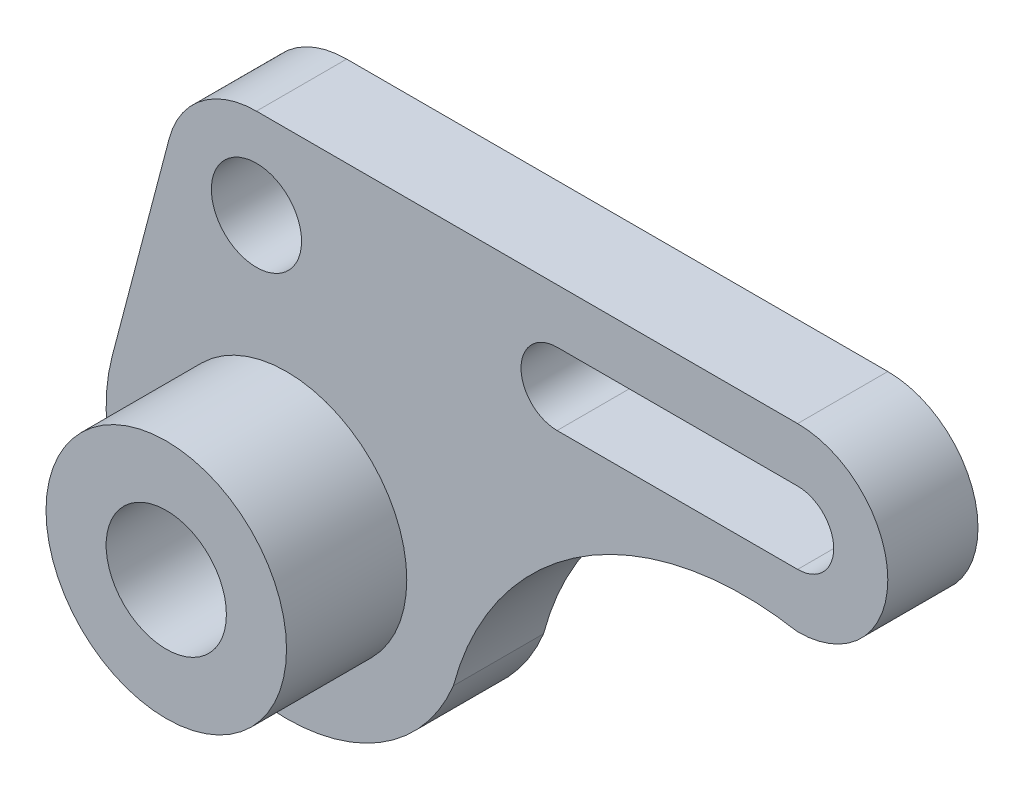
ISO-10303-21;
HEADER;
FILE_DESCRIPTION(('STEP AP214'),'2;1');
FILE_NAME('part.step','',(''),(''),'','','');
FILE_SCHEMA(('AUTOMOTIVE_DESIGN { 1 0 10303 214 1 1 1 1 }'));
ENDSEC;
DATA;
#1=APPLICATION_CONTEXT('core data for automotive mechanical design processes');
#2=APPLICATION_PROTOCOL_DEFINITION('international standard','automotive_design',2000,#1);
#3=PRODUCT_CONTEXT('',#1,'mechanical');
#4=PRODUCT('Part','Part','',(#3));
#5=PRODUCT_RELATED_PRODUCT_CATEGORY('part','',(#4));
#6=PRODUCT_DEFINITION_FORMATION('','',#4);
#7=PRODUCT_DEFINITION_CONTEXT('part definition',#1,'design');
#8=PRODUCT_DEFINITION('design','',#6,#7);
#9=PRODUCT_DEFINITION_SHAPE('','',#8);
#10=(LENGTH_UNIT() NAMED_UNIT(*) SI_UNIT(.MILLI.,.METRE.));
#11=(NAMED_UNIT(*) PLANE_ANGLE_UNIT() SI_UNIT($,.RADIAN.));
#12=(NAMED_UNIT(*) SI_UNIT($,.STERADIAN.) SOLID_ANGLE_UNIT());
#13=UNCERTAINTY_MEASURE_WITH_UNIT(LENGTH_MEASURE(1.E-05),#10,'distance_accuracy_value','');
#14=(GEOMETRIC_REPRESENTATION_CONTEXT(3) GLOBAL_UNCERTAINTY_ASSIGNED_CONTEXT((#13)) GLOBAL_UNIT_ASSIGNED_CONTEXT((#10,
#11,#12)) REPRESENTATION_CONTEXT('',''));
#15=CARTESIAN_POINT('',(0.,0.,0.));
#16=DIRECTION('',(0.,0.,1.));
#17=DIRECTION('',(1.,0.,0.));
#18=AXIS2_PLACEMENT_3D('',#15,#16,#17);
#19=CARTESIAN_POINT('',(105.,-15.,15.));
#20=DIRECTION('',(0.,0.,-1.));
#21=DIRECTION('',(-1.,0.,0.));
#22=AXIS2_PLACEMENT_3D('',#19,#20,#21);
#23=CYLINDRICAL_SURFACE('',#22,15.);
#24=CARTESIAN_POINT('',(105.,-15.,0.));
#25=DIRECTION('',(0.,0.,1.));
#26=DIRECTION('',(1.,0.,0.));
#27=AXIS2_PLACEMENT_3D('',#24,#25,#26);
#28=CIRCLE('',#27,15.);
#29=CARTESIAN_POINT('',(105.,-30.,0.));
#30=VERTEX_POINT('',#29);
#31=CARTESIAN_POINT('',(105.,0.,0.));
#32=VERTEX_POINT('',#31);
#33=EDGE_CURVE('E175',#30,#32,#28,.T.);
#34=ORIENTED_EDGE('',*,*,#33,.T.);
#35=DIRECTION('',(0.,0.,-1.));
#36=VECTOR('',#35,1.);
#37=CARTESIAN_POINT('',(105.,0.,15.));
#38=LINE('',#37,#36);
#39=CARTESIAN_POINT('',(105.,0.,15.));
#40=VERTEX_POINT('',#39);
#41=EDGE_CURVE('E11',#40,#32,#38,.T.);
#42=ORIENTED_EDGE('',*,*,#41,.F.);
#43=CARTESIAN_POINT('',(105.,-15.,15.));
#44=DIRECTION('',(0.,0.,1.));
#45=DIRECTION('',(1.,0.,0.));
#46=AXIS2_PLACEMENT_3D('',#43,#44,#45);
#47=CIRCLE('',#46,15.);
#48=CARTESIAN_POINT('',(105.,-30.,15.));
#49=VERTEX_POINT('',#48);
#50=EDGE_CURVE('E178',#49,#40,#47,.T.);
#51=ORIENTED_EDGE('',*,*,#50,.F.);
#52=DIRECTION('',(0.,0.,-1.));
#53=VECTOR('',#52,1.);
#54=CARTESIAN_POINT('',(105.,-30.,15.));
#55=LINE('',#54,#53);
#56=EDGE_CURVE('E188',#49,#30,#55,.T.);
#57=ORIENTED_EDGE('',*,*,#56,.T.);
#58=EDGE_LOOP('',(#34,#42,#51,#57));
#59=FACE_BOUND('',#58,.T.);
#60=ADVANCED_FACE('F44',(#59),#23,.T.);
#61=CARTESIAN_POINT('',(15.0000000000001,0.,15.));
#62=DIRECTION('',(0.,-1.,0.));
#63=DIRECTION('',(0.,0.,-1.));
#64=AXIS2_PLACEMENT_3D('',#61,#62,#63);
#65=PLANE('',#64);
#66=DIRECTION('',(-1.,0.,0.));
#67=VECTOR('',#66,1.);
#68=CARTESIAN_POINT('',(15.0000000000001,0.,0.));
#69=LINE('',#68,#67);
#70=CARTESIAN_POINT('',(15.0000000000001,0.,0.));
#71=VERTEX_POINT('',#70);
#72=EDGE_CURVE('E191',#32,#71,#69,.T.);
#73=ORIENTED_EDGE('',*,*,#72,.T.);
#74=DIRECTION('',(0.,0.,-1.));
#75=VECTOR('',#74,1.);
#76=CARTESIAN_POINT('',(15.0000000000001,0.,15.));
#77=LINE('',#76,#75);
#78=CARTESIAN_POINT('',(15.0000000000001,0.,15.));
#79=VERTEX_POINT('',#78);
#80=EDGE_CURVE('E55',#79,#71,#77,.T.);
#81=ORIENTED_EDGE('',*,*,#80,.F.);
#82=DIRECTION('',(-1.,0.,0.));
#83=VECTOR('',#82,1.);
#84=CARTESIAN_POINT('',(15.0000000000001,0.,15.));
#85=LINE('',#84,#83);
#86=EDGE_CURVE('E179',#40,#79,#85,.T.);
#87=ORIENTED_EDGE('',*,*,#86,.F.);
#88=ORIENTED_EDGE('',*,*,#41,.T.);
#89=EDGE_LOOP('',(#73,#81,#87,#88));
#90=FACE_BOUND('',#89,.T.);
#91=ADVANCED_FACE('F239',(#90),#65,.F.);
#92=CARTESIAN_POINT('',(15.,-15.,15.));
#93=DIRECTION('',(0.,0.,-1.));
#94=DIRECTION('',(-1.,0.,0.));
#95=AXIS2_PLACEMENT_3D('',#92,#93,#94);
#96=CYLINDRICAL_SURFACE('',#95,15.);
#97=CARTESIAN_POINT('',(15.,-15.,0.));
#98=DIRECTION('',(0.,0.,1.));
#99=DIRECTION('',(1.,0.,0.));
#100=AXIS2_PLACEMENT_3D('',#97,#98,#99);
#101=CIRCLE('',#100,15.);
#102=CARTESIAN_POINT('',(0.492341956526993,-11.1884572554341,0.));
#103=VERTEX_POINT('',#102);
#104=EDGE_CURVE('E192',#71,#103,#101,.T.);
#105=ORIENTED_EDGE('',*,*,#104,.T.);
#106=DIRECTION('',(0.,0.,-1.));
#107=VECTOR('',#106,1.);
#108=CARTESIAN_POINT('',(0.492341956526993,-11.1884572554341,15.));
#109=LINE('',#108,#107);
#110=CARTESIAN_POINT('',(0.492341956526993,-11.1884572554341,15.));
#111=VERTEX_POINT('',#110);
#112=EDGE_CURVE('E209',#111,#103,#109,.T.);
#113=ORIENTED_EDGE('',*,*,#112,.F.);
#114=CARTESIAN_POINT('',(15.,-15.,15.));
#115=DIRECTION('',(0.,0.,1.));
#116=DIRECTION('',(1.,0.,0.));
#117=AXIS2_PLACEMENT_3D('',#114,#115,#116);
#118=CIRCLE('',#117,15.);
#119=EDGE_CURVE('E185',#79,#111,#118,.T.);
#120=ORIENTED_EDGE('',*,*,#119,.F.);
#121=ORIENTED_EDGE('',*,*,#80,.T.);
#122=EDGE_LOOP('',(#105,#113,#120,#121));
#123=FACE_BOUND('',#122,.T.);
#124=ADVANCED_FACE('F220',(#123),#96,.T.);
#125=CARTESIAN_POINT('',(-9.01531608694612,-47.3769145108682,15.));
#126=DIRECTION('',(0.9671772028982,-0.254102849637728,0.));
#127=DIRECTION('',(0.254102849637728,0.9671772028982,0.));
#128=AXIS2_PLACEMENT_3D('',#125,#126,#127);
#129=PLANE('',#128);
#130=DIRECTION('',(-0.254102849637728,-0.9671772028982,0.));
#131=VECTOR('',#130,1.);
#132=CARTESIAN_POINT('',(-9.01531608694612,-47.3769145108682,0.));
#133=LINE('',#132,#131);
#134=CARTESIAN_POINT('',(-9.01531608694612,-47.3769145108682,0.));
#135=VERTEX_POINT('',#134);
#136=EDGE_CURVE('E197',#103,#135,#133,.T.);
#137=ORIENTED_EDGE('',*,*,#136,.T.);
#138=DIRECTION('',(0.,0.,-1.));
#139=VECTOR('',#138,1.);
#140=CARTESIAN_POINT('',(-9.01531608694612,-47.3769145108682,15.));
#141=LINE('',#140,#139);
#142=CARTESIAN_POINT('',(-9.01531608694612,-47.3769145108682,15.));
#143=VERTEX_POINT('',#142);
#144=EDGE_CURVE('E210',#143,#135,#141,.T.);
#145=ORIENTED_EDGE('',*,*,#144,.F.);
#146=DIRECTION('',(-0.254102849637728,-0.9671772028982,0.));
#147=VECTOR('',#146,1.);
#148=CARTESIAN_POINT('',(-9.01531608694612,-47.3769145108682,15.));
#149=LINE('',#148,#147);
#150=EDGE_CURVE('E184',#111,#143,#149,.T.);
#151=ORIENTED_EDGE('',*,*,#150,.F.);
#152=ORIENTED_EDGE('',*,*,#112,.T.);
#153=EDGE_LOOP('',(#137,#145,#151,#152));
#154=FACE_BOUND('',#153,.T.);
#155=ADVANCED_FACE('F229',(#154),#129,.F.);
#156=CARTESIAN_POINT('',(20.,-55.,15.));
#157=DIRECTION('',(0.,0.,-1.));
#158=DIRECTION('',(-1.,0.,0.));
#159=AXIS2_PLACEMENT_3D('',#156,#157,#158);
#160=CYLINDRICAL_SURFACE('',#159,30.);
#161=CARTESIAN_POINT('',(20.,-55.,0.));
#162=DIRECTION('',(0.,0.,1.));
#163=DIRECTION('',(1.,0.,0.));
#164=AXIS2_PLACEMENT_3D('',#161,#162,#163);
#165=CIRCLE('',#164,30.);
#166=CARTESIAN_POINT('',(47.7525615192124,-66.3927753037761,0.));
#167=VERTEX_POINT('',#166);
#168=EDGE_CURVE('E200',#135,#167,#165,.T.);
#169=ORIENTED_EDGE('',*,*,#168,.T.);
#170=DIRECTION('',(0.,0.,-1.));
#171=VECTOR('',#170,1.);
#172=CARTESIAN_POINT('',(47.7525615192124,-66.3927753037761,15.));
#173=LINE('',#172,#171);
#174=CARTESIAN_POINT('',(47.7525615192124,-66.3927753037761,15.));
#175=VERTEX_POINT('',#174);
#176=EDGE_CURVE('E204',#175,#167,#173,.T.);
#177=ORIENTED_EDGE('',*,*,#176,.F.);
#178=CARTESIAN_POINT('',(20.,-55.,15.));
#179=DIRECTION('',(0.,0.,1.));
#180=DIRECTION('',(1.,0.,0.));
#181=AXIS2_PLACEMENT_3D('',#178,#179,#180);
#182=CIRCLE('',#181,30.);
#183=EDGE_CURVE('E187',#143,#175,#182,.T.);
#184=ORIENTED_EDGE('',*,*,#183,.F.);
#185=ORIENTED_EDGE('',*,*,#144,.T.);
#186=EDGE_LOOP('',(#169,#177,#184,#185));
#187=FACE_BOUND('',#186,.T.);
#188=ADVANCED_FACE('F233',(#187),#160,.T.);
#189=CARTESIAN_POINT('',(96.0848114598886,-79.1987745100858,15.));
#190=DIRECTION('',(0.,0.,-1.));
#191=DIRECTION('',(-1.,0.,0.));
#192=AXIS2_PLACEMENT_3D('',#189,#190,#191);
#193=CYLINDRICAL_SURFACE('',#192,50.);
#194=CARTESIAN_POINT('',(96.0848114598886,-79.1987745100858,0.));
#195=DIRECTION('',(0.,0.,-1.));
#196=DIRECTION('',(-1.,0.,0.));
#197=AXIS2_PLACEMENT_3D('',#194,#195,#196);
#198=CIRCLE('',#197,50.);
#199=EDGE_CURVE('E177',#167,#30,#198,.T.);
#200=ORIENTED_EDGE('',*,*,#199,.T.);
#201=ORIENTED_EDGE('',*,*,#56,.F.);
#202=CARTESIAN_POINT('',(96.0848114598886,-79.1987745100858,15.));
#203=DIRECTION('',(0.,0.,-1.));
#204=DIRECTION('',(-1.,0.,0.));
#205=AXIS2_PLACEMENT_3D('',#202,#203,#204);
#206=CIRCLE('',#205,50.);
#207=EDGE_CURVE('E190',#175,#49,#206,.T.);
#208=ORIENTED_EDGE('',*,*,#207,.F.);
#209=ORIENTED_EDGE('',*,*,#176,.T.);
#210=EDGE_LOOP('',(#200,#201,#208,#209));
#211=FACE_BOUND('',#210,.T.);
#212=ADVANCED_FACE('F244',(#211),#193,.F.);
#213=CARTESIAN_POINT('',(105.,-15.,15.));
#214=DIRECTION('',(0.,0.,1.));
#215=DIRECTION('',(1.,0.,0.));
#216=AXIS2_PLACEMENT_3D('',#213,#214,#215);
#217=PLANE('',#216);
#218=CARTESIAN_POINT('',(65.,-15.,15.));
#219=DIRECTION('',(0.,0.,1.));
#220=DIRECTION('',(1.,0.,0.));
#221=AXIS2_PLACEMENT_3D('',#218,#219,#220);
#222=CIRCLE('',#221,6.);
#223=CARTESIAN_POINT('',(65.,-9.,15.));
#224=VERTEX_POINT('',#223);
#225=CARTESIAN_POINT('',(65.,-21.,15.));
#226=VERTEX_POINT('',#225);
#227=EDGE_CURVE('E56',#224,#226,#222,.T.);
#228=ORIENTED_EDGE('',*,*,#227,.F.);
#229=DIRECTION('',(-1.,0.,0.));
#230=VECTOR('',#229,1.);
#231=CARTESIAN_POINT('',(65.,-9.,15.));
#232=LINE('',#231,#230);
#233=CARTESIAN_POINT('',(105.,-9.,15.));
#234=VERTEX_POINT('',#233);
#235=EDGE_CURVE('E139',#234,#224,#232,.T.);
#236=ORIENTED_EDGE('',*,*,#235,.F.);
#237=CARTESIAN_POINT('',(105.,-15.,15.));
#238=DIRECTION('',(0.,0.,1.));
#239=DIRECTION('',(1.,0.,0.));
#240=AXIS2_PLACEMENT_3D('',#237,#238,#239);
#241=CIRCLE('',#240,6.);
#242=CARTESIAN_POINT('',(105.,-21.,15.));
#243=VERTEX_POINT('',#242);
#244=EDGE_CURVE('E142',#243,#234,#241,.T.);
#245=ORIENTED_EDGE('',*,*,#244,.F.);
#246=DIRECTION('',(1.,0.,0.));
#247=VECTOR('',#246,1.);
#248=CARTESIAN_POINT('',(105.,-21.,15.));
#249=LINE('',#248,#247);
#250=EDGE_CURVE('E146',#226,#243,#249,.T.);
#251=ORIENTED_EDGE('',*,*,#250,.F.);
#252=EDGE_LOOP('',(#228,#236,#245,#251));
#253=FACE_BOUND('',#252,.T.);
#254=CARTESIAN_POINT('',(15.,-15.,15.));
#255=DIRECTION('',(0.,0.,1.));
#256=DIRECTION('',(1.,0.,0.));
#257=AXIS2_PLACEMENT_3D('',#254,#255,#256);
#258=CIRCLE('',#257,7.5);
#259=CARTESIAN_POINT('',(22.5,-15.,15.));
#260=VERTEX_POINT('',#259);
#261=EDGE_CURVE('E152',#260,#260,#258,.T.);
#262=ORIENTED_EDGE('',*,*,#261,.F.);
#263=EDGE_LOOP('',(#262));
#264=FACE_BOUND('',#263,.T.);
#265=CARTESIAN_POINT('',(20.,-55.,15.));
#266=DIRECTION('',(0.,0.,1.));
#267=DIRECTION('',(1.,0.,0.));
#268=AXIS2_PLACEMENT_3D('',#265,#266,#267);
#269=CIRCLE('',#268,20.);
#270=CARTESIAN_POINT('',(40.,-55.,15.));
#271=VERTEX_POINT('',#270);
#272=EDGE_CURVE('E170',#271,#271,#269,.T.);
#273=ORIENTED_EDGE('',*,*,#272,.F.);
#274=EDGE_LOOP('',(#273));
#275=FACE_BOUND('',#274,.T.);
#276=ORIENTED_EDGE('',*,*,#50,.T.);
#277=ORIENTED_EDGE('',*,*,#86,.T.);
#278=ORIENTED_EDGE('',*,*,#119,.T.);
#279=ORIENTED_EDGE('',*,*,#150,.T.);
#280=ORIENTED_EDGE('',*,*,#183,.T.);
#281=ORIENTED_EDGE('',*,*,#207,.T.);
#282=EDGE_LOOP('',(#276,#277,#278,#279,#280,#281));
#283=FACE_BOUND('',#282,.T.);
#284=ADVANCED_FACE('F232',(#253,#264,#275,#283),#217,.T.);
#285=CARTESIAN_POINT('',(105.,-15.,0.));
#286=DIRECTION('',(0.,0.,1.));
#287=DIRECTION('',(1.,0.,0.));
#288=AXIS2_PLACEMENT_3D('',#285,#286,#287);
#289=PLANE('',#288);
#290=DIRECTION('',(-1.,0.,0.));
#291=VECTOR('',#290,1.);
#292=CARTESIAN_POINT('',(65.,-9.,0.));
#293=LINE('',#292,#291);
#294=CARTESIAN_POINT('',(105.,-9.,0.));
#295=VERTEX_POINT('',#294);
#296=CARTESIAN_POINT('',(65.,-9.,0.));
#297=VERTEX_POINT('',#296);
#298=EDGE_CURVE('E129',#295,#297,#293,.T.);
#299=ORIENTED_EDGE('',*,*,#298,.T.);
#300=CARTESIAN_POINT('',(65.,-15.,0.));
#301=DIRECTION('',(0.,0.,1.));
#302=DIRECTION('',(1.,0.,0.));
#303=AXIS2_PLACEMENT_3D('',#300,#301,#302);
#304=CIRCLE('',#303,6.);
#305=CARTESIAN_POINT('',(65.,-21.,0.));
#306=VERTEX_POINT('',#305);
#307=EDGE_CURVE('E121',#297,#306,#304,.T.);
#308=ORIENTED_EDGE('',*,*,#307,.T.);
#309=DIRECTION('',(1.,0.,0.));
#310=VECTOR('',#309,1.);
#311=CARTESIAN_POINT('',(105.,-21.,0.));
#312=LINE('',#311,#310);
#313=CARTESIAN_POINT('',(105.,-21.,0.));
#314=VERTEX_POINT('',#313);
#315=EDGE_CURVE('E134',#306,#314,#312,.T.);
#316=ORIENTED_EDGE('',*,*,#315,.T.);
#317=CARTESIAN_POINT('',(105.,-15.,0.));
#318=DIRECTION('',(0.,0.,1.));
#319=DIRECTION('',(1.,0.,0.));
#320=AXIS2_PLACEMENT_3D('',#317,#318,#319);
#321=CIRCLE('',#320,6.);
#322=EDGE_CURVE('E70',#314,#295,#321,.T.);
#323=ORIENTED_EDGE('',*,*,#322,.T.);
#324=EDGE_LOOP('',(#299,#308,#316,#323));
#325=FACE_BOUND('',#324,.T.);
#326=CARTESIAN_POINT('',(15.,-15.,0.));
#327=DIRECTION('',(0.,0.,1.));
#328=DIRECTION('',(1.,0.,0.));
#329=AXIS2_PLACEMENT_3D('',#326,#327,#328);
#330=CIRCLE('',#329,7.5);
#331=CARTESIAN_POINT('',(22.5,-15.,0.));
#332=VERTEX_POINT('',#331);
#333=EDGE_CURVE('E158',#332,#332,#330,.T.);
#334=ORIENTED_EDGE('',*,*,#333,.T.);
#335=EDGE_LOOP('',(#334));
#336=FACE_BOUND('',#335,.T.);
#337=CARTESIAN_POINT('',(20.,-55.,0.));
#338=DIRECTION('',(0.,0.,1.));
#339=DIRECTION('',(1.,0.,0.));
#340=AXIS2_PLACEMENT_3D('',#337,#338,#339);
#341=CIRCLE('',#340,10.);
#342=CARTESIAN_POINT('',(30.,-55.,0.));
#343=VERTEX_POINT('',#342);
#344=EDGE_CURVE('E163',#343,#343,#341,.T.);
#345=ORIENTED_EDGE('',*,*,#344,.T.);
#346=EDGE_LOOP('',(#345));
#347=FACE_BOUND('',#346,.T.);
#348=ORIENTED_EDGE('',*,*,#33,.F.);
#349=ORIENTED_EDGE('',*,*,#199,.F.);
#350=ORIENTED_EDGE('',*,*,#168,.F.);
#351=ORIENTED_EDGE('',*,*,#136,.F.);
#352=ORIENTED_EDGE('',*,*,#104,.F.);
#353=ORIENTED_EDGE('',*,*,#72,.F.);
#354=EDGE_LOOP('',(#348,#349,#350,#351,#352,#353));
#355=FACE_BOUND('',#354,.T.);
#356=ADVANCED_FACE('F138',(#325,#336,#347,#355),#289,.F.);
#357=CARTESIAN_POINT('',(20.,-55.,35.));
#358=DIRECTION('',(0.,0.,-1.));
#359=DIRECTION('',(-1.,0.,0.));
#360=AXIS2_PLACEMENT_3D('',#357,#358,#359);
#361=CYLINDRICAL_SURFACE('',#360,20.);
#362=CARTESIAN_POINT('',(20.,-55.,35.));
#363=DIRECTION('',(0.,0.,1.));
#364=DIRECTION('',(1.,0.,0.));
#365=AXIS2_PLACEMENT_3D('',#362,#363,#364);
#366=CIRCLE('',#365,20.);
#367=CARTESIAN_POINT('',(40.,-55.,35.));
#368=VERTEX_POINT('',#367);
#369=EDGE_CURVE('E168',#368,#368,#366,.T.);
#370=ORIENTED_EDGE('',*,*,#369,.F.);
#371=EDGE_LOOP('',(#370));
#372=FACE_BOUND('',#371,.T.);
#373=ORIENTED_EDGE('',*,*,#272,.T.);
#374=EDGE_LOOP('',(#373));
#375=FACE_BOUND('',#374,.T.);
#376=ADVANCED_FACE('F315',(#372,#375),#361,.T.);
#377=CARTESIAN_POINT('',(20.,-55.,35.));
#378=DIRECTION('',(0.,0.,1.));
#379=DIRECTION('',(1.,0.,0.));
#380=AXIS2_PLACEMENT_3D('',#377,#378,#379);
#381=PLANE('',#380);
#382=CARTESIAN_POINT('',(20.,-55.,35.));
#383=DIRECTION('',(0.,0.,1.));
#384=DIRECTION('',(1.,0.,0.));
#385=AXIS2_PLACEMENT_3D('',#382,#383,#384);
#386=CIRCLE('',#385,10.);
#387=CARTESIAN_POINT('',(30.,-55.,35.));
#388=VERTEX_POINT('',#387);
#389=EDGE_CURVE('E161',#388,#388,#386,.T.);
#390=ORIENTED_EDGE('',*,*,#389,.F.);
#391=EDGE_LOOP('',(#390));
#392=FACE_BOUND('',#391,.T.);
#393=ORIENTED_EDGE('',*,*,#369,.T.);
#394=EDGE_LOOP('',(#393));
#395=FACE_BOUND('',#394,.T.);
#396=ADVANCED_FACE('F312',(#392,#395),#381,.T.);
#397=CARTESIAN_POINT('',(20.,-55.,0.));
#398=DIRECTION('',(0.,0.,1.));
#399=DIRECTION('',(1.,0.,0.));
#400=AXIS2_PLACEMENT_3D('',#397,#398,#399);
#401=CYLINDRICAL_SURFACE('',#400,10.);
#402=ORIENTED_EDGE('',*,*,#344,.F.);
#403=EDGE_LOOP('',(#402));
#404=FACE_BOUND('',#403,.T.);
#405=ORIENTED_EDGE('',*,*,#389,.T.);
#406=EDGE_LOOP('',(#405));
#407=FACE_BOUND('',#406,.T.);
#408=ADVANCED_FACE('F325',(#404,#407),#401,.F.);
#409=CARTESIAN_POINT('',(15.,-15.,0.));
#410=DIRECTION('',(0.,0.,1.));
#411=DIRECTION('',(1.,0.,0.));
#412=AXIS2_PLACEMENT_3D('',#409,#410,#411);
#413=CYLINDRICAL_SURFACE('',#412,7.5);
#414=ORIENTED_EDGE('',*,*,#333,.F.);
#415=EDGE_LOOP('',(#414));
#416=FACE_BOUND('',#415,.T.);
#417=ORIENTED_EDGE('',*,*,#261,.T.);
#418=EDGE_LOOP('',(#417));
#419=FACE_BOUND('',#418,.T.);
#420=ADVANCED_FACE('F329',(#416,#419),#413,.F.);
#421=CARTESIAN_POINT('',(65.,-15.,0.));
#422=DIRECTION('',(0.,0.,1.));
#423=DIRECTION('',(1.,0.,0.));
#424=AXIS2_PLACEMENT_3D('',#421,#422,#423);
#425=CYLINDRICAL_SURFACE('',#424,6.);
#426=ORIENTED_EDGE('',*,*,#227,.T.);
#427=DIRECTION('',(0.,0.,1.));
#428=VECTOR('',#427,1.);
#429=CARTESIAN_POINT('',(65.,-21.,0.));
#430=LINE('',#429,#428);
#431=EDGE_CURVE('E116',#306,#226,#430,.T.);
#432=ORIENTED_EDGE('',*,*,#431,.F.);
#433=ORIENTED_EDGE('',*,*,#307,.F.);
#434=DIRECTION('',(0.,0.,1.));
#435=VECTOR('',#434,1.);
#436=CARTESIAN_POINT('',(65.,-9.,0.));
#437=LINE('',#436,#435);
#438=EDGE_CURVE('E155',#297,#224,#437,.T.);
#439=ORIENTED_EDGE('',*,*,#438,.T.);
#440=EDGE_LOOP('',(#426,#432,#433,#439));
#441=FACE_BOUND('',#440,.T.);
#442=ADVANCED_FACE('F123',(#441),#425,.F.);
#443=CARTESIAN_POINT('',(65.,-9.,0.));
#444=DIRECTION('',(0.,1.,0.));
#445=DIRECTION('',(0.,0.,1.));
#446=AXIS2_PLACEMENT_3D('',#443,#444,#445);
#447=PLANE('',#446);
#448=ORIENTED_EDGE('',*,*,#235,.T.);
#449=ORIENTED_EDGE('',*,*,#438,.F.);
#450=ORIENTED_EDGE('',*,*,#298,.F.);
#451=DIRECTION('',(0.,0.,1.));
#452=VECTOR('',#451,1.);
#453=CARTESIAN_POINT('',(105.,-9.,0.));
#454=LINE('',#453,#452);
#455=EDGE_CURVE('E154',#295,#234,#454,.T.);
#456=ORIENTED_EDGE('',*,*,#455,.T.);
#457=EDGE_LOOP('',(#448,#449,#450,#456));
#458=FACE_BOUND('',#457,.T.);
#459=ADVANCED_FACE('F342',(#458),#447,.F.);
#460=CARTESIAN_POINT('',(105.,-15.,0.));
#461=DIRECTION('',(0.,0.,1.));
#462=DIRECTION('',(1.,0.,0.));
#463=AXIS2_PLACEMENT_3D('',#460,#461,#462);
#464=CYLINDRICAL_SURFACE('',#463,6.);
#465=ORIENTED_EDGE('',*,*,#244,.T.);
#466=ORIENTED_EDGE('',*,*,#455,.F.);
#467=ORIENTED_EDGE('',*,*,#322,.F.);
#468=DIRECTION('',(0.,0.,1.));
#469=VECTOR('',#468,1.);
#470=CARTESIAN_POINT('',(105.,-21.,0.));
#471=LINE('',#470,#469);
#472=EDGE_CURVE('E126',#314,#243,#471,.T.);
#473=ORIENTED_EDGE('',*,*,#472,.T.);
#474=EDGE_LOOP('',(#465,#466,#467,#473));
#475=FACE_BOUND('',#474,.T.);
#476=ADVANCED_FACE('F354',(#475),#464,.F.);
#477=CARTESIAN_POINT('',(105.,-21.,0.));
#478=DIRECTION('',(0.,-1.,0.));
#479=DIRECTION('',(0.,0.,-1.));
#480=AXIS2_PLACEMENT_3D('',#477,#478,#479);
#481=PLANE('',#480);
#482=ORIENTED_EDGE('',*,*,#250,.T.);
#483=ORIENTED_EDGE('',*,*,#472,.F.);
#484=ORIENTED_EDGE('',*,*,#315,.F.);
#485=ORIENTED_EDGE('',*,*,#431,.T.);
#486=EDGE_LOOP('',(#482,#483,#484,#485));
#487=FACE_BOUND('',#486,.T.);
#488=ADVANCED_FACE('F135',(#487),#481,.F.);
#489=CLOSED_SHELL('',(#60,#91,#124,#155,#188,#212,#284,#356,#376,#396,#408,#420,#442,#459,#476,#488));
#490=MANIFOLD_SOLID_BREP('B2',#489);
#491=ADVANCED_BREP_SHAPE_REPRESENTATION('',(#18,#490),#14);
#492=SHAPE_DEFINITION_REPRESENTATION(#9,#491);
ENDSEC;
END-ISO-10303-21;
